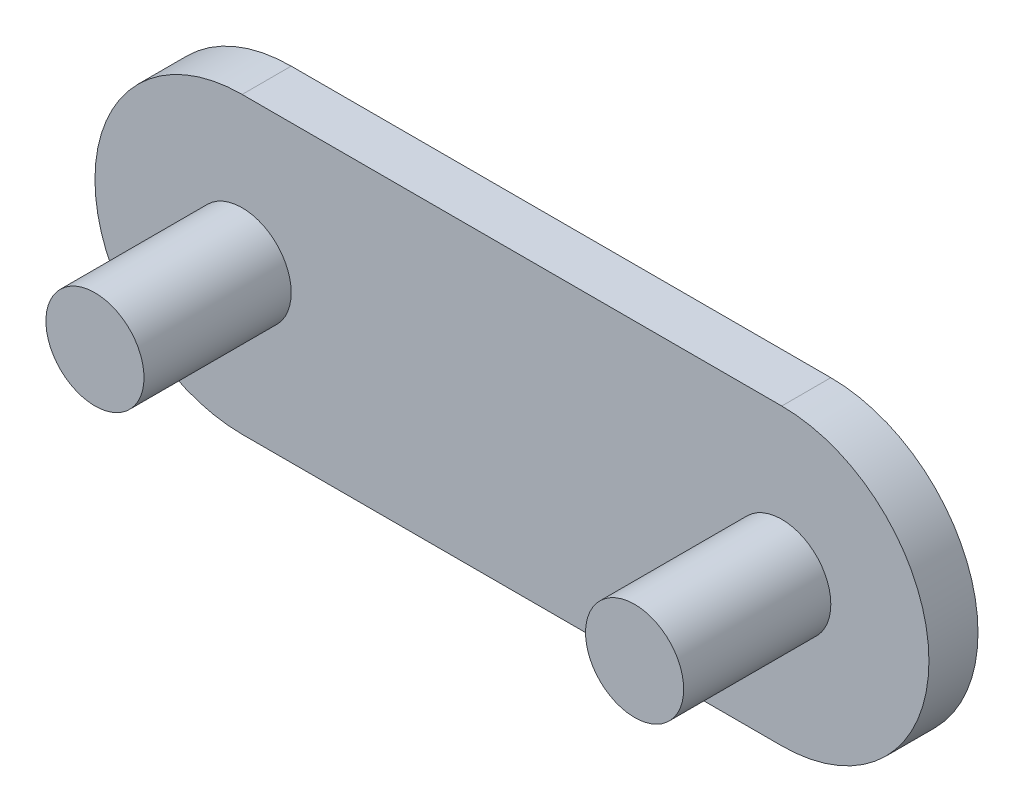
SolidWorks part; units mm, degrees
material "Plain Carbon Steel"
ref_plane "Front Plane" through (0, 0, 0) normal (0, 0, 1) x (1, 0, 0)
ref_plane "Top Plane" through (0, 0, 0) normal (0, 1, 0) x (1, 0, 0)
ref_plane "Right Plane" through (0, 0, 0) normal (1, 0, 0) x (0, 0, -1)
sketch "Plate Outline Sketch" plane through (0, 0, 0) normal (0, 0, 1) x (1, 0, 0)
  line L0 (-27.5, 0) -> (27.5, 0) construction
  line L1 (-27.5, 15) -> (27.5, 15)
  line L2 (-27.5, -15) -> (27.5, -15)
  arc A0 (-27.5, 15) -> (-27.5, -15) centre (-27.5, 0) ccw
  arc A1 (27.5, -15) -> (27.5, 15) centre (27.5, 0) ccw
  point P3 (0, 0)
  dimension "D1" = 15
  dimension "D2" = 55
extrude "Base Plate" add sketch "Plate Outline Sketch" along normal blind 5
sketch "Pin Circles Sketch" plane through (0, 0, 5) normal (0, 0, 1) x (1, 0, 0)
  circle A0 centre (-27.5, 0) radius 5
  circle A1 centre (27.5, 0) radius 5
  dimension "D1" = 10
  dimension "D2" = 10
extrude "Pins 2xØ10" add sketch "Pin Circles Sketch" along normal blind 15
